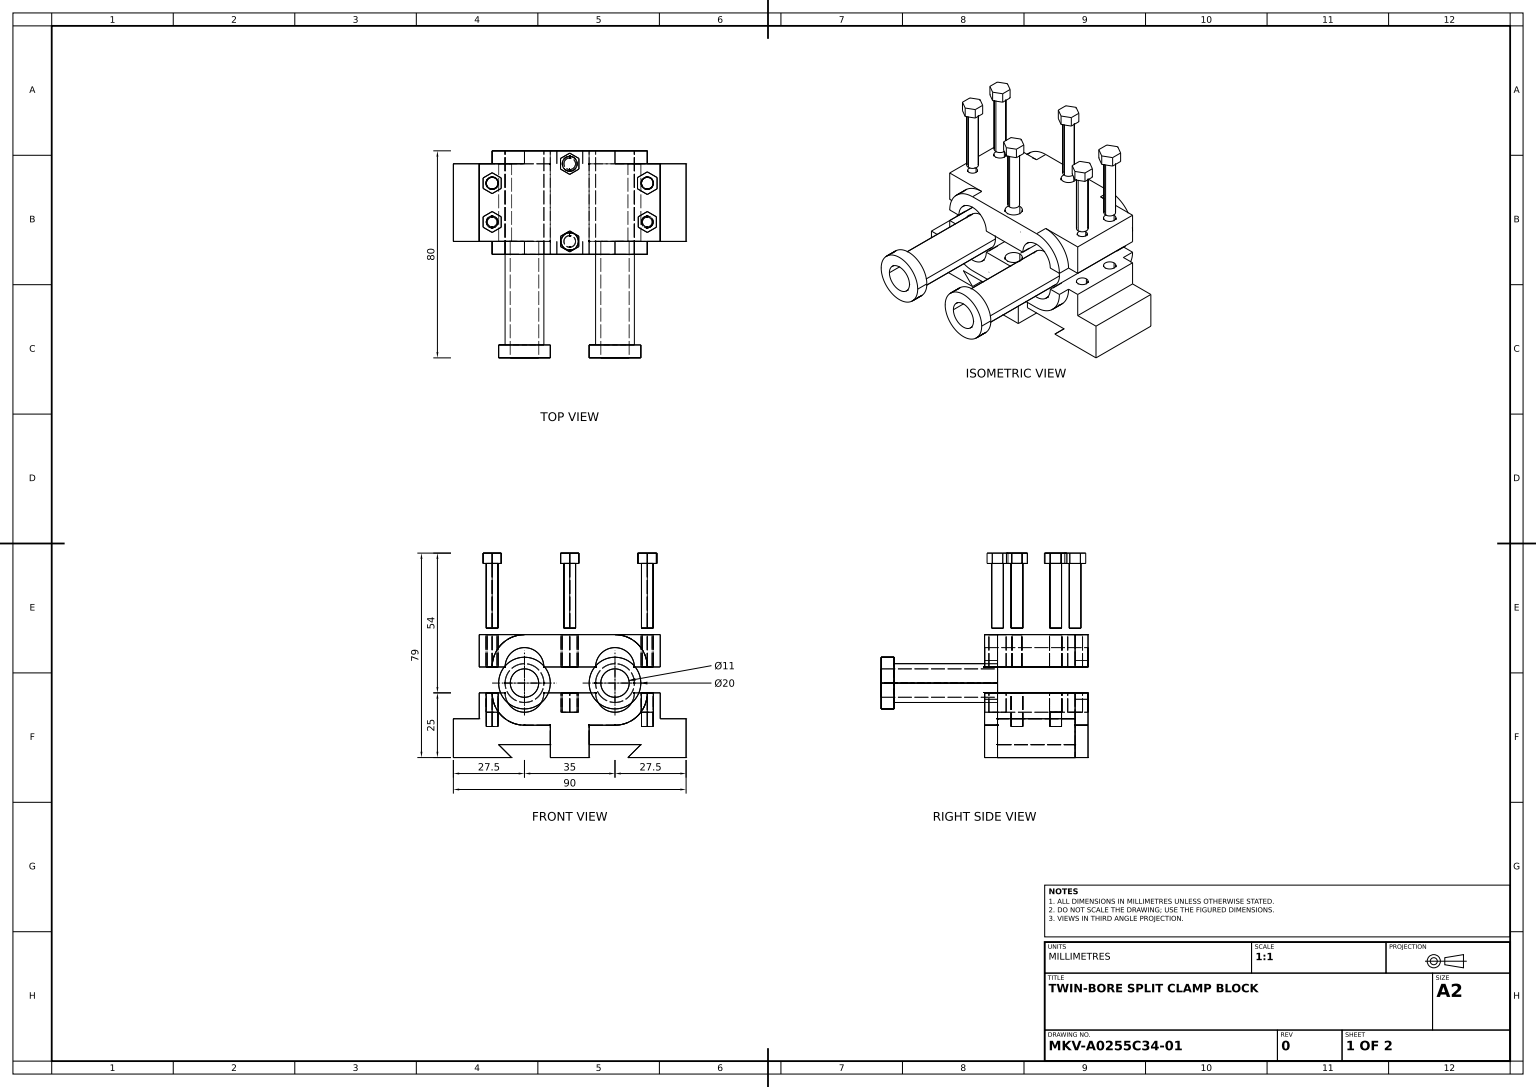
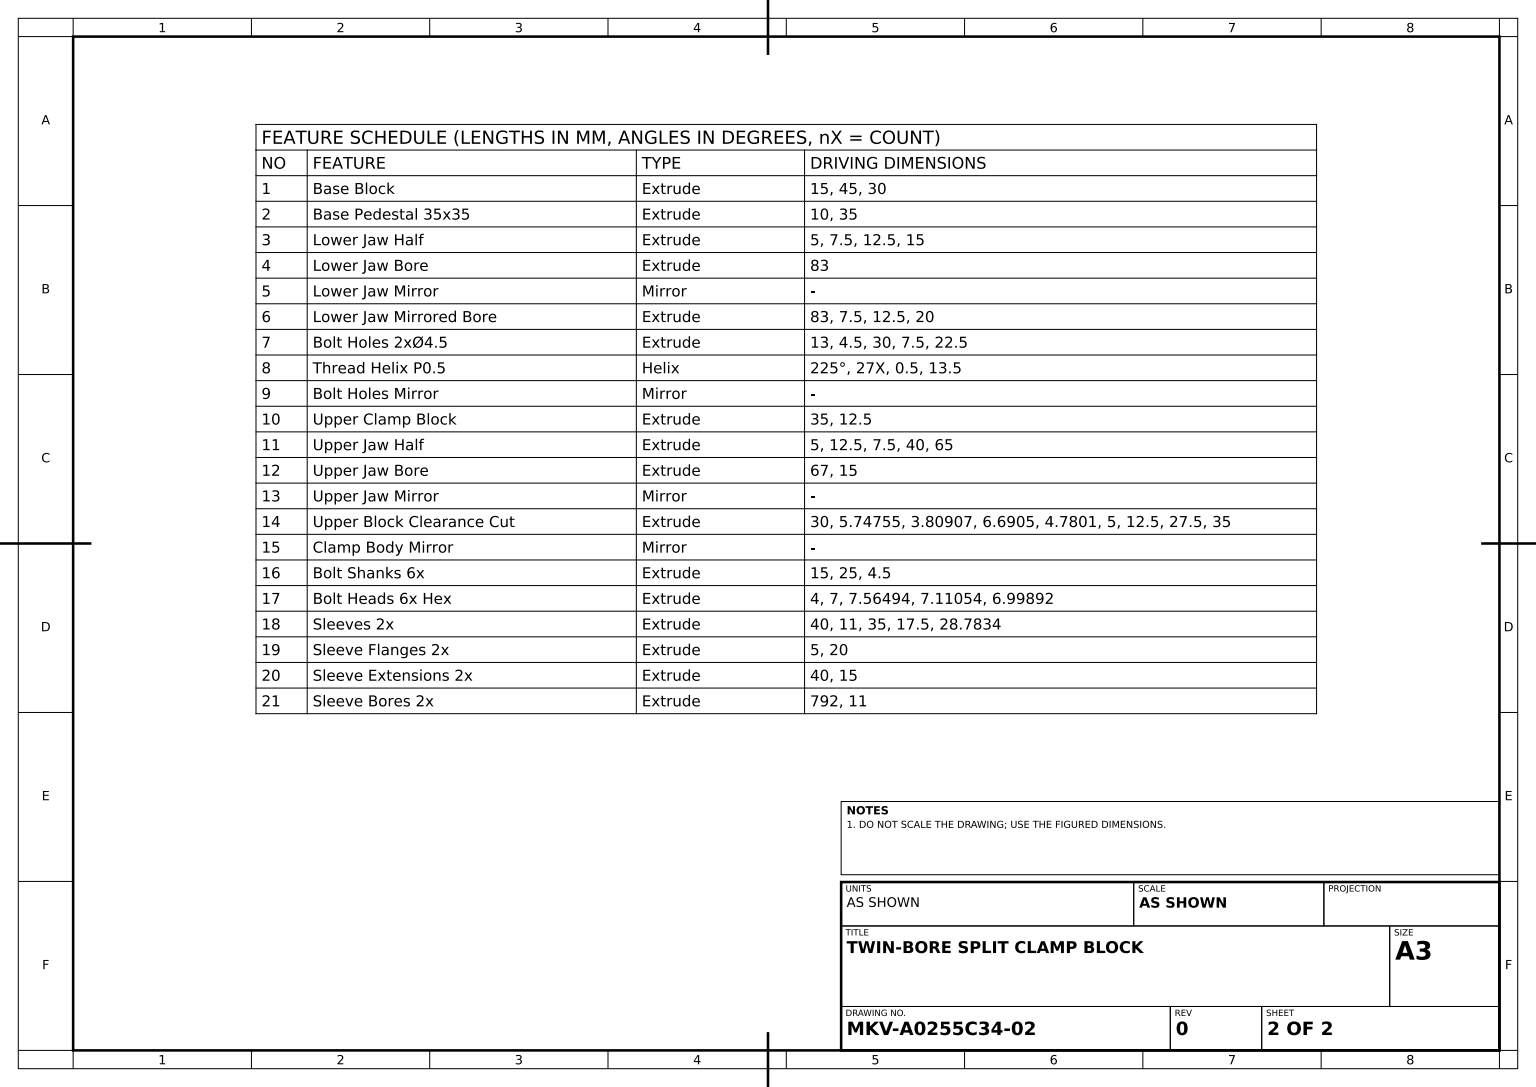
SolidWorks part; units mm, degrees
material "Plain Carbon Steel"
ref_plane "Front Plane" through (0, 0, 0) normal (0, 0, 1) x (1, 0, 0)
ref_plane "Top Plane" through (0, 0, 0) normal (0, 1, 0) x (1, 0, 0)
ref_plane "Right Plane" through (0, 0, 0) normal (1, 0, 0) x (0, 0, -1)
sketch "Base Block Sketch" plane through (0, 0, 0) normal (0, 1, 0) x (1, 0, 0)
  line L0 (0, 0) -> (45, 0)
  line L1 (0, 0) -> (-45, 0)
  line L2 (-45, 0) -> (-45, 30)
  line L3 (-45, 30) -> (45, 30)
  line L4 (45, 30) -> (45, 0)
  dimension "D1" = 45
  dimension "D2" = 45
  dimension "D3" = 30
extrude "Base Block" add sketch "Base Block Sketch" along normal blind 15
sketch "Base Pedestal Sketch" plane through (0, 15, 0) normal (0, 1, 0) x (1, 0, 0)
  line L1 (-45, 0) -> (45, 0) construction
  line L2 (-35, 0) -> (-35, 30)
  line L3 (45, 30) -> (-45, 30) construction
  line L4 (-35, 30) -> (35, 30)
  line L5 (35, 30) -> (35, 0)
  line L6 (35, 0) -> (-35, 0)
  dimension "D1" = 35
  dimension "D2" = 35
extrude "Base Pedestal 35x35" add sketch "Base Pedestal Sketch" along normal blind 10
sketch "Lower Jaw Sketch" plane through (0, 0, 0) normal (0, 0, 1) x (1, 0, 0)
  line L0 (-35, 25) -> (-17.5, 25)
  line L1 (-35, 25) -> (35, 25) construction
  line L2 (0, 0) -> (-7.5, 0)
  line L3 (-45, 0) -> (45, 0) construction
  line L4 (-7.5, 0) -> (-7.5, 12.5)
  line L5 (-7.5, 12.5) -> (-17.5, 12.5)
  line L6 (-17.5, 25) -> (-10, 25)
  line L7 (-30, 25) -> (30, 25)
  line L8 (0, 0) -> (7.5, 0)
  line L9 (7.5, 0) -> (7.5, 12.5)
  line L10 (7.5, 12.5) -> (17.5, 12.5)
  line L11 (30, 25) -> (25, 25)
  line L12 (10, 25) -> (17.5, 25)
  line L13 (45, 15) -> (45, 0) construction
  arc A0 (-25, 25) -> (-10, 25) centre (-17.5, 25) ccw
  arc A1 (-30, 25) -> (-17.5, 12.5) centre (-17.5, 25) ccw
  arc A2 (10, 25) -> (25, 25) centre (17.5, 25) ccw
  arc A3 (17.5, 12.5) -> (30, 25) centre (17.5, 25) ccw
  line M11 (-45, 0) -> (45, 0)
  line M15 (35, 25) -> (-35, 25)
  dimension "D1" = 7.5
  dimension "D2" = 12.5
  dimension "D3" = 15
extrude "Lower Jaw Half" add sketch "Lower Jaw Sketch" along normal blind 5 contours L10 A3 A2 L7 A0 A1 L5 L4 L9 M15 M11
sketch "Lower Jaw Bore Sketch" plane through (0, 0, 5) normal (0, 0, 1) x (1, 0, 0)
  line L0 (-25, 25) -> (-10, 25) construction
  line L1 (10, 25) -> (25, 25) construction
  circle A0 centre (-17.5, 25) radius 7.5
  circle A1 centre (17.5, 25) radius 7.5
extrude "Lower Jaw Bore" cut sketch "Lower Jaw Bore Sketch" against normal blind 83
ref_plane "Plane1" through (0, 0, -15) normal (0, 0, 1) x (1, 0, 0)
mirror "Lower Jaw Mirror" about plane through (0, 0, -15) normal (0, 0, 1) of "Lower Jaw Half"
sketch "Lower Jaw Mirrored Bore Sketch" plane through (0, 0, -30) normal (0, 0, -1) x (-1, 0, 0)
  line L0 (-22.5, 0) -> (22.5, 0)
  line L1 (7.5, 0) -> (45, 0) construction
  line L4 (27.5, 5) -> (22.5, 0)
  line L5 (0, 0) -> (0, 25)
  line L6 (-10, 25) -> (10, 25) construction
  line L7 (-27.5, 5) -> (-22.5, 0)
  line L8 (-27.5, 5) -> (27.5, 5)
  line L9 (7.5, 0) -> (7.5, 5)
  line L10 (7.5, 0) -> (7.5, 12.5) construction
  line L11 (7.5, 5) -> (-7.5, 5)
  line L12 (-7.5, 0) -> (-7.5, 12.5) construction
  line L13 (-7.5, 5) -> (-7.5, 0)
  line L14 (-7.5, 0) -> (7.5, 0)
  line L15 (-35, 25) -> (-35, 15) construction
  line L16 (-35, 25) -> (-30, 25) construction
  line M14 (-45, 0) -> (-7.5, 0)
  line M15 (-7.5, 0) -> (-7.5, 12.5)
  dimension "D1" = 7.5
  dimension "D2" = 12.5
  dimension "D3" = 20
extrude "Lower Jaw Mirrored Bore" cut sketch "Lower Jaw Mirrored Bore Sketch" against normal blind 83 contours L8 L7 M14 M15 | L9 L0 L4 L8
sketch "Bolt Holes Sketch" plane through (0, 25, 0) normal (0, 1, 0) x (1, 0, 0)
  circle A0 centre (30, 7.5) radius 2.25
  circle A1 centre (30, 22.5) radius 2.25
  dimension "D1" = 4.5
  dimension "D2" = 4.5
  dimension "D3" = 30
  dimension "D4" = 7.5
  dimension "D5" = 30
  dimension "D6" = 22.5
extrude "Bolt Holes 2xØ4.5" cut sketch "Bolt Holes Sketch" against normal blind 13
sketch "Thread Helix Sketch" plane through (0, 25, 0) normal (0, 1, 0) x (1, 0, 0)
  circle A0 centre (30, 7.5) radius 2.25
  dimension "D1" = 4.5
curve "Thread Helix P0.5" pitch 0.5 height 13.5 turns 27
mirror "Bolt Holes Mirror" about plane through (0, 0, 0) normal (1, 0, 0) of "Bolt Holes 2xØ4.5"
ref_plane "Plane2" through (0, 35, 0) normal (0, 1, 0) x (1, 0, 0)
sketch "Upper Clamp Block Sketch" plane through (0, 35, 0) normal (0, 1, 0) x (1, 0, 0)
  line L0 (-35, 0) -> (-35, 30)
  line L1 (-35, 30) -> (35, 30)
  line L2 (35, 30) -> (35, 0)
  line L3 (35, 0) -> (-35, 0)
extrude "Upper Clamp Block" add sketch "Upper Clamp Block Sketch" along normal blind 12.5 separate body
sketch "Upper Jaw Sketch" plane through (0, 0, 0) normal (0, 0, 1) x (1, 0, 0)
  line L0 (22, 35) -> (-22, 35) construction
  line L1 (-30, 35) -> (-5, 35)
  line L2 (5, 35) -> (30, 35)
  line L3 (-5, 35) -> (5, 35)
  line L4 (-17.5, 47.5) -> (17.5, 47.5)
  line L5 (35, 47.5) -> (35, 35) construction
  arc A0 (-17.5, 47.5) -> (-30, 35) centre (-17.5, 35) ccw
  arc A1 (-10, 35) -> (-25, 35) centre (-17.5, 35) ccw
  arc A2 (30, 35) -> (17.5, 47.5) centre (17.5, 35) ccw
  arc A3 (25, 35) -> (10, 35) centre (17.5, 35) ccw
  line M7 (-35, 35) -> (35, 35)
  line M9 (35, 47.5) -> (-35, 47.5)
  dimension "D1" = 12.5
  dimension "D2" = 7.5
  dimension "D3" = 5
  dimension "D4" = 40
  dimension "D5" = 65
extrude "Upper Jaw Half" add sketch "Upper Jaw Sketch" along normal blind 5 contours A3 A2 A0 A1 M7 M9
sketch "Upper Jaw Bore Sketch" plane through (0, 0, 5) normal (0, 0, 1) x (1, 0, 0)
  circle A0 centre (-17.5, 35) radius 7.5
  circle A1 centre (17.5, 35) radius 7.5
  dimension "D1" = 15
extrude "Upper Jaw Bore" cut sketch "Upper Jaw Bore Sketch" against normal blind 67
mirror "Upper Jaw Mirror" about plane through (0, 0, -15) normal (0, 0, 1) of "Upper Jaw Half"
sketch "Upper Block Clearance Sketch" plane through (0, 47.5, 0) normal (0, 1, 0) x (1, 0, 0)
  line L0 (35, 0) -> (35, 30) construction
  line L1 (17.5, -5) -> (-17.5, -5) construction
  circle A0 centre (30, 22.5) radius 2.3901
  circle A1 centre (30, 7.5) radius 1.9045
  circle A2 centre (0, 30) radius 2.8738
  circle A3 centre (0, 0) radius 3.3453
  dimension "D1" = 5.7475
  dimension "D2" = 3.8091
  dimension "D3" = 6.6905
  dimension "D4" = 4.7801
  dimension "D5" = 5
  dimension "D6" = 12.5
  dimension "D7" = 27.5
  dimension "D8" = 35
extrude "Upper Block Clearance Cut" cut sketch "Upper Block Clearance Sketch" against normal blind 30
mirror "Clamp Body Mirror" about plane through (0, 0, 0) normal (1, 0, 0) of "Upper Block Clearance Cut"
ref_plane "Plane3" through (0, 50, 0) normal (0, 1, 0) x (1, 0, 0)
sketch "Bolt Shanks Sketch" plane through (0, 50, 0) normal (0, 1, 0) x (1, 0, 0)
  circle A0 centre (0, 0) radius 2.25
  circle A1 centre (30, 22.5) radius 2.25
  circle A2 centre (30, 7.5) radius 2.25
  circle A3 centre (0, 30) radius 2.25
  circle A4 centre (-30, 7.5) radius 2.25
  circle A5 centre (-30, 22.5) radius 2.25
  dimension "D1" = 4.5
extrude "Bolt Shanks 6x" add sketch "Bolt Shanks Sketch" along normal blind 25 separate body
sketch "Bolt Heads Sketch" plane through (0, 75, 0) normal (0, 1, 0) x (1, 0, 0)
  line L1 (0, 34.1053) -> (-3.5553, 32.0526)
  line L2 (-3.5553, 32.0526) -> (-3.5553, 27.9474)
  line L3 (-3.5553, 27.9474) -> (0, 25.8947)
  line L4 (0, 25.8947) -> (3.5553, 27.9474)
  line L5 (3.5553, 27.9474) -> (3.5553, 32.0526)
  line L6 (3.5553, 32.0526) -> (0, 34.1053)
  line L7 (0, 4.0415) -> (-3.5, 2.0207)
  line L8 (-3.5, 2.0207) -> (-3.5, -2.0207)
  line L9 (-3.5, -2.0207) -> (0, -4.0415)
  line L10 (0, -4.0415) -> (3.5, -2.0207)
  line L11 (3.5, -2.0207) -> (3.5, 2.0207)
  line L12 (3.5, 2.0207) -> (0, 4.0415)
  line L13 (30, 26.8676) -> (26.2175, 24.6838)
  line L14 (26.2175, 24.6838) -> (26.2175, 20.3162)
  line L15 (26.2175, 20.3162) -> (30, 18.1324)
  line L16 (30, 18.1324) -> (33.7825, 20.3162)
  line L17 (33.7825, 20.3162) -> (33.7825, 24.6838)
  line L18 (33.7825, 24.6838) -> (30, 26.8676)
  line L19 (30, 11.5408) -> (26.5005, 9.5204)
  line L20 (26.5005, 9.5204) -> (26.5005, 5.4796)
  line L21 (26.5005, 5.4796) -> (30, 3.4592)
  line L22 (30, 3.4592) -> (33.4995, 5.4796)
  line L23 (33.4995, 5.4796) -> (33.4995, 9.5204)
  line L24 (33.4995, 9.5204) -> (30, 11.5408)
  line L25 (-30, 26.5415) -> (-33.5, 24.5207)
  line L26 (-33.5, 24.5207) -> (-33.5, 20.4793)
  line L27 (-33.5, 20.4793) -> (-30, 18.4585)
  line L28 (-30, 18.4585) -> (-26.5, 20.4793)
  line L29 (-26.5, 20.4793) -> (-26.5, 24.5207)
  line L30 (-26.5, 24.5207) -> (-30, 26.5415)
  line L31 (-30, 11.5415) -> (-33.5, 9.5207)
  line L32 (-33.5, 9.5207) -> (-33.5, 5.4793)
  line L33 (-33.5, 5.4793) -> (-30, 3.4585)
  line L34 (-30, 3.4585) -> (-26.5, 5.4793)
  line L35 (-26.5, 5.4793) -> (-26.5, 9.5207)
  line L36 (-26.5, 9.5207) -> (-30, 11.5415)
  circle A0 centre (0, 30) radius 3.5553 construction
  circle A1 centre (0, 0) radius 3.5 construction
  circle A2 centre (30, 22.5) radius 3.7825 construction
  circle A3 centre (30, 7.5) radius 3.4995 construction
  circle A4 centre (-30, 22.5) radius 3.5 construction
  circle A5 centre (-30, 7.5) radius 3.5 construction
  dimension "D1" = 7
  dimension "D2" = 7.5649
  dimension "D3" = 7.1105
  dimension "D4" = 6.9989
extrude "Bolt Heads 6x Hex" add sketch "Bolt Heads Sketch" along normal blind 4
sketch "Sleeves Sketch" plane through (0, 0, 0) normal (0, 0, 1) x (1, 0, 0)
  circle A0 centre (-17.5, 28.7834) radius 5.5
  circle A1 centre (17.5, 28.7834) radius 5.5
  dimension "D1" = 11
  dimension "D2" = 35
  dimension "D3" = 17.5
  dimension "D4" = 28.7834
extrude "Sleeves 2x" add sketch "Sleeves Sketch" along normal blind 40 separate body
sketch "Sleeve Flanges Sketch" plane through (0, 0, 40) normal (0, 0, 1) x (1, 0, 0)
  circle A1 centre (-17.5, 28.7834) radius 10
  circle A2 centre (17.5, 28.7834) radius 10
  dimension "D1" = 20
extrude "Sleeve Flanges 2x" add sketch "Sleeve Flanges Sketch" along normal blind 5
sketch "Sleeve Extensions Sketch" plane through (0, 0, 0) normal (0, 0, -1) x (-1, 0, 0)
  circle A0 centre (-17.5, 28.7834) radius 7.5
  circle A1 centre (17.5, 28.7834) radius 7.5
  dimension "D1" = 15
extrude "Sleeve Extensions 2x" add sketch "Sleeve Extensions Sketch" against normal blind 40
sketch "Sleeve Bores Sketch" plane through (0, 0, 45) normal (0, 0, 1) x (1, 0, 0)
  circle A0 centre (-17.5, 28.7834) radius 5.5
  circle A1 centre (17.5, 28.7834) radius 5.5
  dimension "D1" = 11
extrude "Sleeve Bores 2x" cut sketch "Sleeve Bores Sketch" against normal blind 792
